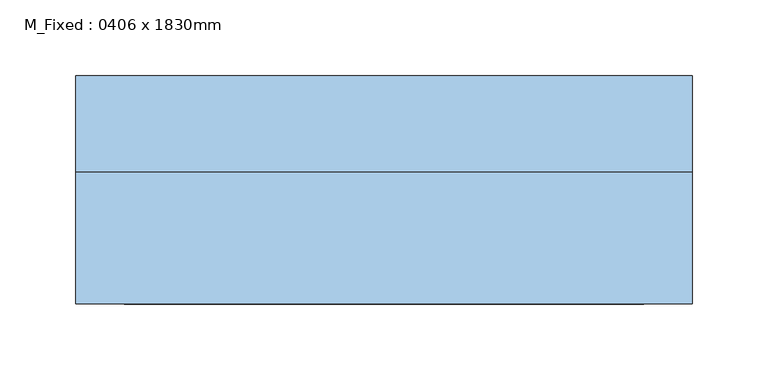
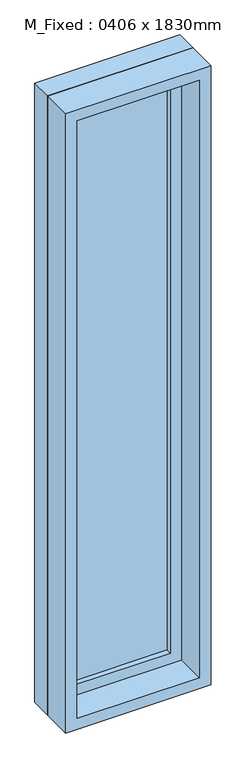
"""IFC4 building model written with IfcOpenShell, lengths in millimetres: window geometry, M_Fixed : 0406 x 1830mm."""

from ifc_helpers import new_model, si_unit, frame, origin, place, context, project, spatial, polyline, outline, extrude, source, transform, mapped, element, save


def m_fixed_0406_x_1830mm_a81fa326(model_context):
    return source(origin(), model_context, "Body", "SweptSolid", [
        extrude(outline(polyline([(-140.0, 53.0), (140.0, 53.0), (140.0, 41.0), (-140.0, 41.0), (-140.0, 53.0)])), frame((0.0, 0.0, 368.0), z_axis=(0.0, 0.0, 1.0), x_axis=(1.0, 0.0, 0.0)), (0.0, 0.0, 1.0), 1704.0),
        extrude(outline(polyline([(2116.0, -184.0), (324.0, -184.0), (324.0, 184.0), (2116.0, 184.0), (2116.0, -184.0)]), holes=[polyline([(2072.0, -140.0), (2072.0, 140.0), (368.0, 140.0), (368.0, -140.0), (2072.0, -140.0)])]), frame((0.0, 25.0, 0.0), z_axis=(0.0, 1.0, 0.0), x_axis=(0.0, 0.0, 1.0)), (0.0, 0.0, 1.0), 44.0),
        extrude(outline(polyline([(2135.0, -203.0), (305.0, -203.0), (305.0, 203.0), (2135.0, 203.0), (2135.0, -203.0)]), holes=[polyline([(2116.0, -184.0), (2116.0, 184.0), (324.0, 184.0), (324.0, -184.0), (2116.0, -184.0)])]), frame((0.0, 25.0, 0.0), z_axis=(0.0, 1.0, 0.0), x_axis=(0.0, 0.0, 1.0)), (0.0, 0.0, 1.0), 63.0),
        extrude(outline(polyline([(2135.0, -203.0), (305.0, -203.0), (305.0, 203.0), (2135.0, 203.0), (2135.0, -203.0)]), holes=[polyline([(2103.0, -171.0), (2103.0, 171.0), (337.0, 171.0), (337.0, -171.0), (2103.0, -171.0)])]), frame((0.0, -62.0, 0.0), z_axis=(0.0, 1.0, 0.0), x_axis=(0.0, 0.0, 1.0)), (0.0, 0.0, 1.0), 87.0),
    ])


if __name__ == "__main__":
    model = new_model("IFC4")
    model_context = context("Model", 3, world=origin())
    ifc_project = project(units=[si_unit("LENGTHUNIT", "METRE", prefix="MILLI")], contexts=[model_context])
    site = spatial("IfcSite", under=ifc_project)
    building = spatial("IfcBuilding", under=site)
    placement = place(None, origin())
    m_fixed_0406_x_1830mm_shape = m_fixed_0406_x_1830mm_a81fa326(model_context)
    element("IfcWindow", 1, ObjectType="M_Fixed : 0406 x 1830mm", at=placement, inside=building, context=model_context, shape_type="MappedRepresentation", body=[
        mapped(m_fixed_0406_x_1830mm_shape, transform((0.0, 0.0, 0.0), x_axis=(1.0, 0.0, 0.0), y_axis=(0.0, 1.0, 0.0), z_axis=(0.0, 0.0, 1.0))),
    ])
    save(model, "model.ifc")

# Revit data of these elements
# Type "M_Fixed : 0406 x 1830mm"
#   Type Mark = "16"
#   Height = 1830 mm
#   Default Sill Height = 305 mm
#   Width = 406 mm
#   Window Inset = 19 mm
#   Frame Exterior Material = Sash
#   Frame Interior Material = Sash
#   Glass Pane Material = Glass
#   Sash = Sash
#   Wall Closure = (empty or 0)
# Element 1 (IfcWindow, "M_Fixed : 0406 x 1830mm")
#   Materials on its faces: "Sash", "Glass"
# Materials
#   "Sash": class "Wood", colour RGB 136 99 55, transparency 0
#   "Glass": class "Glass", colour RGB 218 227 224, transparency 0.85, Description = "Soda Lime Glass", Cost = 0
